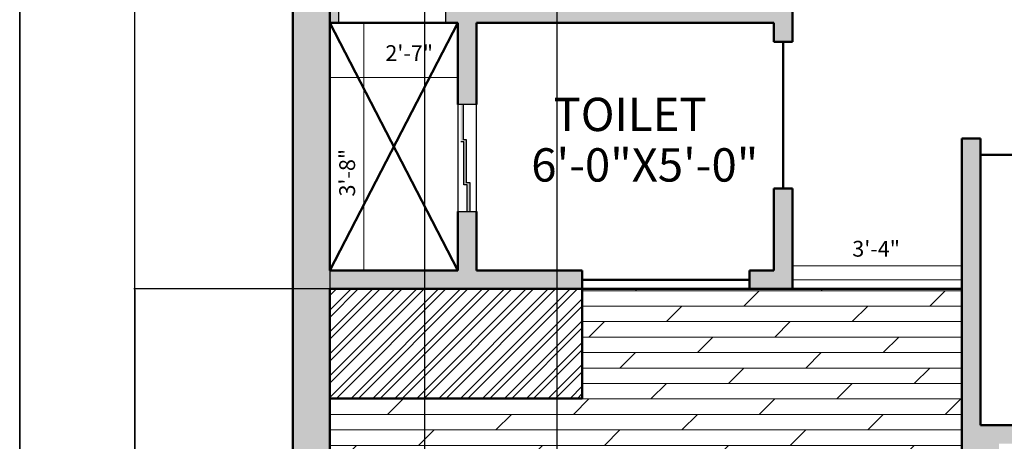
# Model space of a CAD drawing. Units: inches. Extents: x 1381 to 2246, y 1317 to 2168.
# Tile 3 of 15: x 1381 to 1619, y 1673 to 1776. Entities that reach past the tile are written whole.
import ezdxf

# ---------------------------------------------------------------- set-up
doc = ezdxf.new("R2010")
doc.units = ezdxf.units.IN
doc.header["$MEASUREMENT"] = 0
for name, color, linetype, lineweight in [('A-ANNO-DIMS', 2, 'Continuous', 18), ('A-ANNO-TEXT', 7, 'Continuous', 18), ('A-ANNO-TTLB', 7, 'Continuous', 35), ('A-AREA-IDEN', 3, 'Continuous', 25), ('A-FLOR-PATT', 252, 'Continuous', 13), ('A-GLAZ', 4, 'Continuous', 25), ('A-WALL', 7, 'Continuous', 50)]:
    doc.layers.add(name, color=color, linetype=linetype, lineweight=lineweight)
doc.styles.get("Standard").update_dxf_attribs({"font": 'arial.ttf'})
doc.dimstyles.get("Standard").update_dxf_attribs({"dimtxt": 7, "dimasz": 0.18, "dimexe": 0.18, "dimexo": 0.0625, "dimgap": 0.09, "dimtad": 0, "dimtih": 1, "dimtoh": 1, "dimdec": 1, "dimzin": 0, "dimdsep": 46, "dimlunit": 3, "dimtxsty": 'Standard', "dimcen": 0.09, "dimadec": 0, "dimazin": 0, "dimtfac": 1, "dimtdec": 1, "dimtofl": 0, "dimtmove": 0, "dimatfit": 3, "dimfxl": 1, "dimtolj": 1, "dimtzin": 0, "dimarcsym": 0})

# ---------------------------------------------------------------- blocks, each defined once
blk = doc.blocks.new('*D50')
at = {"layer": 'A-ANNO-DIMS', "color": 0, "lineweight": -2, "transparency": 16777216}
for p, q in [((1446.99, 2092.92), (1408.62, 2092.92)), ((1408.8, 2092.74), (1408.8, 1786.08)), ((1408.8, 1472.1), (1408.8, 1778.75)), ((1446.99, 1471.92), (1408.62, 1471.92))]:
    blk.add_line(p, q, dxfattribs=at)
at = {"layer": 'A-ANNO-DIMS', "color": 0, "transparency": 16777216}
for points in [[(1408.77, 2092.74), (1408.83, 2092.74), (1408.8, 2092.92)], [(1408.77, 1472.1), (1408.83, 1472.1), (1408.8, 1471.92)]]:
    blk.add_solid(points, dxfattribs=at)
at = {"layer": 'Defpoints', "color": 0, "transparency": 16777216}
for p in [(1408.8, 2092.92), (1447.05, 2092.92), (1447.05, 1471.92)]:
    blk.add_point(p, dxfattribs=at)
at = {"layer": 'A-ANNO-DIMS', "color": 0, "transparency": 16777216, "insert": (1408.8, 1782.42), "char_height": 7, "attachment_point": 5}
blk.add_mtext('\\A1;621', dxfattribs=at)
blk = doc.blocks.new('*D55')
at = {"layer": 'A-ANNO-DIMS', "color": 0, "lineweight": -2, "transparency": 16777216}
for p, q in [((1455.99, 1710.42), (1408.62, 1710.42)), ((1408.8, 1710.24), (1408.8, 1648.08)), ((1408.8, 1578.6), (1408.8, 1640.75)), ((1455.99, 1578.42), (1408.62, 1578.42))]:
    blk.add_line(p, q, dxfattribs=at)
at = {"layer": 'A-ANNO-DIMS', "color": 0, "transparency": 16777216}
for points in [[(1408.77, 1710.24), (1408.83, 1710.24), (1408.8, 1710.42)], [(1408.77, 1578.6), (1408.83, 1578.6), (1408.8, 1578.42)]]:
    blk.add_solid(points, dxfattribs=at)
at = {"layer": 'Defpoints', "color": 0, "transparency": 16777216}
for p in [(1408.8, 1710.42), (1456.05, 1710.42), (1456.05, 1578.42)]:
    blk.add_point(p, dxfattribs=at)
at = {"layer": 'A-ANNO-DIMS', "color": 0, "transparency": 16777216, "insert": (1408.8, 1644.42), "char_height": 7, "attachment_point": 5}
blk.add_mtext('\\A1;132', dxfattribs=at)
blk = doc.blocks.new('*D67')
at = {"layer": 'A-ANNO-DIMS', "color": 0, "lineweight": -2, "transparency": 16777216}
for p, q in [((1456.050973, 1911.353813), (1456.050973, 1384.360695)), ((1478.962127, 1911.353813), (1478.962127, 1384.360695)), ((1455.870973, 1384.540695), (1455.690973, 1384.540695)), ((1479.142127, 1384.540695), (1479.322127, 1384.540695))]:
    blk.add_line(p, q, dxfattribs=at)
at = {"layer": 'A-ANNO-DIMS', "color": 0, "transparency": 16777216}
for points in [[(1455.870973, 1384.570695), (1455.870973, 1384.510695), (1456.050973, 1384.540695)], [(1479.142127, 1384.570695), (1479.142127, 1384.510695), (1478.962127, 1384.540695)]]:
    blk.add_solid(points, dxfattribs=at)
at = {"layer": 'Defpoints', "color": 0, "transparency": 16777216}
for p in [(1456.050973, 1911.416313), (1478.962127, 1911.416313), (1478.962127, 1384.540695)]:
    blk.add_point(p, dxfattribs=at)
at = {"layer": 'A-ANNO-DIMS', "color": 0, "transparency": 16777216, "insert": (1467.50655, 1384.540695), "char_height": 7, "attachment_point": 5}
blk.add_mtext('\\A1;22.91', dxfattribs=at)
blk = doc.blocks.new('*D68')
at = {"layer": 'A-ANNO-DIMS', "color": 0, "lineweight": -2, "transparency": 16777216}
for p, q in [((1478.96, 1911.35), (1478.96, 1384.36)), ((1511.02, 1911.35), (1511.02, 1384.36)), ((1479.14, 1384.54), (1480.39, 1384.54)), ((1510.84, 1384.54), (1509.59, 1384.54))]:
    blk.add_line(p, q, dxfattribs=at)
at = {"layer": 'A-ANNO-DIMS', "color": 0, "transparency": 16777216}
for points in [[(1479.14, 1384.57), (1479.14, 1384.51), (1478.96, 1384.54)], [(1510.84, 1384.57), (1510.84, 1384.51), (1511.02, 1384.54)]]:
    blk.add_solid(points, dxfattribs=at)
at = {"layer": 'Defpoints', "color": 0, "transparency": 16777216}
for p in [(1478.96, 1911.42), (1511.02, 1911.42), (1511.02, 1384.54)]:
    blk.add_point(p, dxfattribs=at)
at = {"layer": 'A-ANNO-DIMS', "color": 0, "transparency": 16777216, "insert": (1494.99, 1384.54), "char_height": 7, "attachment_point": 5}
blk.add_mtext('\\A1;32.054', dxfattribs=at)

msp = doc.modelspace()

# ---------------------------------------------------------------- hatches: boundary and pattern name
at = {"layer": 'A-FLOR-PATT'}
h = msp.add_hatch(dxfattribs=at)
h.set_pattern_fill('ANSI32', color=256, scale=10)
h.paths.add_polyline_path([(1517.1194, 1710.4163), (1456.051, 1710.4163), (1456.051, 1683.9148), (1517.1194, 1683.9148)])
h = msp.add_hatch(dxfattribs=at)
h.set_pattern_fill('DOLMIT', color=256, scale=15)
h.paths.add_polyline_path([(1609.051, 1710.4163), (1517.1194, 1710.4163), (1517.1194, 1683.9148), (1456.051, 1683.9148), (1456.051, 1578.4163), (1545.7088, 1578.4163), (1609.051, 1578.4163)])
h.paths.add_polyline_path([(1528.374, 1667.7293), (1528.374, 1599.2474), (1499.8186, 1599.2474), (1499.8186, 1606.0382), (1473.6909, 1606.0382), (1473.8019, 1594.5315), (1460.606, 1594.5315), (1460.4951, 1606.0382), (1460.4951, 1657.3975), (1460.3841, 1668.9042), (1473.5799, 1668.9042), (1473.6909, 1657.3975), (1499.8186, 1657.3975), (1499.8186, 1667.7293)], flags=16)
h.paths.add_polyline_path([(1478.0548, 1657.3422), (1478.0548, 1648.0757), (1471.2225, 1648.0757), (1471.1765, 1648.0133), (1471.1765, 1611.8376), (1463.4157, 1611.8376), (1463.4157, 1626.8866), (1471.1765, 1626.8866), (1471.1765, 1633.0267), (1463.4157, 1633.0267), (1463.4157, 1648.0757), (1471.2225, 1648.0757)], flags=0)
h.paths.add_polyline_path([(1471.2297, 1663.4608, -1), (1462.7343, 1663.4608, -1)], flags=0)
h.paths.add_polyline_path([(1471.3407, 1600.5947, -1), (1462.8453, 1600.5947, -1)], flags=0)
h.paths.add_polyline_path([(1534.4824, 1621.5603), (1603.5976, 1621.5603), (1603.5976, 1633.9282), (1534.4824, 1633.9282)], flags=24)
h.paths.add_polyline_path([(1528.6332, 1634.5998), (1609.2654, 1634.5998), (1609.2654, 1647.1329), (1528.6332, 1647.1329)], flags=9)
h.paths.add_polyline_path([(1534.0271, 1646.8395), (1599.6229, 1646.8395), (1599.6229, 1659.3726), (1534.0271, 1659.3726)], flags=24)
at = {"layer": 'A-GLAZ'}
h = msp.add_hatch(color=256, dxfattribs=at)
h.dxf.hatch_style = 1
h.paths.add_polyline_path([(1456.051, 2083.9163), (1737.551, 2083.9163), (1737.551, 1677.4163), (1732.8596, 1677.4163), (1732.8596, 1672.9163), (1737.551, 1672.9163), (1737.551, 1471.9163), (1746.551, 1471.9163), (1746.551, 2092.9163), (1447.051, 2092.9163), (1447.051, 2083.9163), (1447.051, 1471.9163), (1488.6632, 1471.9163), (1488.6632, 1480.9163), (1456.051, 1480.9163), (1456.051, 1710.4163), (1517.1194, 1710.4163), (1517.1194, 1714.9163), (1491.551, 1714.9163), (1491.551, 1729.193), (1487.051, 1729.193), (1487.051, 1714.9163), (1456.051, 1714.9163)])
h.paths.add_polyline_path([(1622.551, 2035.4163), (1625.0954, 2035.4163), (1625.0954, 2039.9163), (1618.051, 2039.9163), (1618.051, 1915.9163), (1611.2353, 1915.9163), (1611.2353, 1911.4163), (1626.5102, 1911.4163), (1626.5102, 1915.9163), (1622.551, 1915.9163)], flags=17)
h.paths.add_polyline_path([(1737.551, 1915.9163), (1668.5102, 1915.9163), (1668.5102, 1911.4163), (1737.551, 1911.4163)], flags=17)
h.paths.add_polyline_path([(1682.2831, 2039.9163), (1655.8191, 2039.9163), (1655.8191, 2035.4163), (1682.2831, 2035.4163)], flags=17)
h.paths.add_polyline_path([(1737.551, 2039.9163), (1725.9636, 2039.9163), (1725.9636, 2035.4163), (1737.551, 2035.4163)], flags=17)
h.paths.add_polyline_path([(1684.2508, 1711.4667), (1740.8192, 1711.4667), (1740.8192, 1723.8346), (1684.2508, 1723.8346)], flags=25)
h = msp.add_hatch(color=256, dxfattribs=at)
h.dxf.hatch_style = 1
h.paths.add_polyline_path([(1478.9621, 1915.9163), (1456.051, 1915.9163), (1456.051, 1911.4163), (1478.9621, 1911.4163)])
h.paths.add_polyline_path([(1566.2107, 1915.9163), (1511.016, 1915.9163), (1511.016, 1911.4163), (1516.051, 1911.4163), (1516.051, 1779.4163), (1484.0852, 1779.4163), (1484.0852, 1774.9163), (1487.051, 1774.9163), (1487.051, 1755.1129), (1491.551, 1755.1129), (1491.551, 1774.9163), (1563.551, 1774.9163), (1563.551, 1770.3401), (1568.051, 1770.3401), (1568.051, 1779.4163), (1520.551, 1779.4163), (1520.551, 1911.4163), (1566.2107, 1911.4163)])
h.paths.add_polyline_path([(1568.051, 1734.7997), (1563.551, 1734.7997), (1563.551, 1714.9163), (1557.5961, 1714.9163), (1557.5961, 1710.4163), (1568.051, 1710.4163)])
h.paths.add_polyline_path([(1458.1653, 1779.4163), (1456.051, 1779.4163), (1456.051, 1774.9163), (1458.1653, 1774.9163)])
h.paths.add_polyline_path([(1684.551, 1746.8536), (1680.051, 1746.8536), (1680.051, 1677.4163), (1673.5117, 1677.4163), (1673.5117, 1672.9163), (1699.1735, 1672.9163), (1699.1735, 1677.4163), (1684.551, 1677.4163)])
h.paths.add_polyline_path([(1613.551, 1746.8536), (1609.051, 1746.8536), (1609.051, 1624.2465), (1618.051, 1624.2465), (1618.051, 1672.9163), (1625.5117, 1672.9163), (1625.5117, 1677.4163), (1613.551, 1677.4163)])
h.paths.add_polyline_path([(1618.051, 1585.1257), (1609.051, 1585.1257), (1609.051, 1569.4163), (1618.051, 1569.4163)])
h.paths.add_polyline_path([(1545.7088, 1578.4163), (1456.051, 1578.4163), (1456.051, 1569.4163), (1545.7088, 1569.4163)])
h.paths.add_polyline_path([(1594.0453, 1480.9163), (1536.6467, 1480.9163), (1536.6467, 1471.9163), (1594.0453, 1471.9163)])
h = msp.add_hatch(color=256, dxfattribs=at)
h.dxf.hatch_style = 1
h.paths.add_polyline_path([(1489.1251, 1736.1591), (1489.1251, 1746.5538), (1488.399, 1746.5538), (1488.399, 1755.1129), (1487.739, 1755.1129), (1487.739, 1746.1133), (1488.5091, 1746.1133), (1488.5091, 1735.6746), (1489.301, 1735.6746), (1489.301, 1729.193), (1490.0272, 1729.193), (1490.0272, 1736.1591)])

# ---------------------------------------------------------------- linework, layer by layer
at = {"layer": 'A-ANNO-DIMS'}
for p, q in [((1464.2798, 1714.9163), (1464.2798, 1774.9163)), ((1456.051, 1761.653), (1487.051, 1761.653)), ((1568.051, 1716.0149), (1609.051, 1716.0149)), ((1568.051, 1712.6663), (1609.051, 1712.6663))]:
    msp.add_line(p, q, dxfattribs=at)
at = {"layer": 'A-ANNO-TTLB'}
msp.add_line((1380.9518, 1316.7761), (1380.9518, 2167.8236), dxfattribs=at)
at = {"layer": 'A-GLAZ'}
for p, q in [((1458.1653, 1779.4163), (1458.1653, 1774.9163)), ((1484.0852, 1774.9163), (1484.0852, 1779.4163)), ((1458.1653, 1774.9163), (1484.0852, 1774.9163)), ((1491.551, 1755.1129), (1487.051, 1755.1129)), ((1487.051, 1755.1129), (1487.051, 1729.193)), ((1488.399, 1746.5538), (1488.399, 1755.1129)), ((1491.551, 1729.193), (1491.551, 1755.1129)), ((1488.5091, 1746.1133), (1487.739, 1746.1133)), ((1489.1251, 1746.5538), (1488.399, 1746.5538)), ((1488.5091, 1735.6746), (1488.5091, 1746.1133)), ((1489.1251, 1736.1591), (1489.1251, 1746.5538)), ((1489.301, 1735.6746), (1488.5091, 1735.6746)), ((1490.0272, 1736.1591), (1489.1251, 1736.1591)), ((1489.301, 1729.193), (1489.301, 1735.6746)), ((1490.0272, 1729.193), (1490.0272, 1736.1591)), ((1487.051, 1729.193), (1491.551, 1729.193)), ((1489.4142, 1729.193), (1489.4142, 1729.193)), ((1490.0272, 1729.193), (1490.0272, 1729.193))]:
    msp.add_line(p, q, dxfattribs=at)
at = {"layer": 'A-WALL'}
for p, q in [((1447.051, 2083.9163), (1447.051, 1471.9163)), ((1456.051, 2083.9163), (1456.051, 1714.9163)), ((1568.051, 1779.4163), (1568.051, 1770.3401)), ((1456.051, 1774.9163), (1487.051, 1774.9163)), ((1487.051, 1714.9163), (1456.051, 1774.9163)), ((1456.051, 1714.9163), (1487.051, 1774.9163)), ((1487.051, 1774.9163), (1487.051, 1755.1129)), ((1491.551, 1774.9163), (1491.551, 1755.1129)), ((1491.551, 1774.9163), (1563.551, 1774.9163)), ((1563.551, 1774.9163), (1563.551, 1770.3401)), ((1563.551, 1770.3401), (1568.051, 1770.3401)), ((1565.801, 1734.7997), (1565.801, 1770.3401)), ((1609.051, 1746.8536), (1609.051, 1569.4163)), ((1613.551, 1746.8536), (1609.051, 1746.8536)), ((1613.551, 1746.8536), (1613.551, 1677.4163)), ((1613.551, 1742.952), (1680.051, 1742.952)), ((1563.551, 1734.7997), (1568.051, 1734.7997)), ((1563.551, 1734.7997), (1563.551, 1714.9163)), ((1568.051, 1734.7997), (1568.051, 1710.4163)), ((1487.051, 1729.193), (1487.051, 1714.9163)), ((1491.551, 1729.193), (1491.551, 1714.9163)), ((1456.051, 1714.9163), (1487.051, 1714.9163)), ((1491.551, 1714.9163), (1517.1194, 1714.9163)), ((1517.1194, 1714.9163), (1517.1194, 1710.4163)), ((1557.5961, 1714.9163), (1557.5961, 1710.4163)), ((1557.5961, 1714.9163), (1563.551, 1714.9163)), ((1557.5961, 1712.6663), (1517.1194, 1712.6663)), ((1456.051, 1710.4163), (1609.051, 1710.4163)), ((1456.051, 1710.4163), (1456.051, 1480.9163)), ((1517.1194, 1710.4163), (1517.1194, 1683.9148)), ((1517.1194, 1683.9148), (1456.051, 1683.9148)), ((1613.551, 1677.4163), (1625.5117, 1677.4163))]:
    msp.add_line(p, q, dxfattribs=at)

# ---------------------------------------------------------------- texts
at = {"layer": 'A-ANNO-TEXT'}
for s, p in [('2\'-7"', (1469.4735, 1765.6616)), ('3\'-4"', (1582.5048, 1718.2494))]:
    msp.add_text(s, height=3.83139, dxfattribs=at).set_placement(p)
msp.add_text('3\'-8"', height=3.83139, rotation=90, dxfattribs=at).set_placement((1462.1406, 1732.8218))
at = {"layer": 'A-AREA-IDEN'}
for s, height, p in [('TOILET', 8.07451, (1510.1818, 1748.6827)), ('6\'-0"X5\'-0"', 8.074511, (1504.7878, 1736.4431))]:
    msp.add_text(s, height=height, dxfattribs=at).set_placement(p)

# ---------------------------------------------------------------- dimensions: what is measured, and where the dimension line sits
at = {"layer": 'A-ANNO-DIMS'}
for base, p1, p2, picture, middle in [((1408.801, 2092.9163), (1447.051, 1471.9163), (1447.051, 2092.9163), '*D50', (1408.801, 1782.4163)), ((1408.801, 1710.4163), (1456.051, 1578.4163), (1456.051, 1710.4163), '*D55', (1408.801, 1644.4163))]:
    dim = msp.add_linear_dim(base=base, p1=p1, p2=p2, angle=90, dimstyle='Standard', override={"dimdec": 0, "dimlfac": 1, "dimrnd": 0, "dimzin": 0, "dimdsep": 46, "dimlunit": 2}, dxfattribs=at)
    dim.commit()
    dim.dimension.update_dxf_attribs({"geometry": picture, "text_midpoint": middle})
for base, p1, p2, override, picture, middle in [((1478.9621, 1384.5407), (1456.051, 1911.4163), (1478.9621, 1911.4163), {"dimdec": 2, "dimlfac": 1, "dimrnd": 0, "dimzin": 0, "dimdsep": 46, "dimlunit": 2}, '*D67', (1467.5066, 1384.5407)), ((1511.016, 1384.5407), (1478.9621, 1911.4163), (1511.016, 1911.4163), {"dimdec": 3, "dimlfac": 1, "dimrnd": 0, "dimzin": 0, "dimdsep": 46, "dimlunit": 2}, '*D68', (1494.9891, 1384.5407))]:
    dim = msp.add_linear_dim(base=base, p1=p1, p2=p2, dimstyle='Standard', override=override, dxfattribs=at)
    dim.commit()
    dim.dimension.update_dxf_attribs({"geometry": picture, "text_midpoint": middle})

doc.saveas('drawing.dxf')
